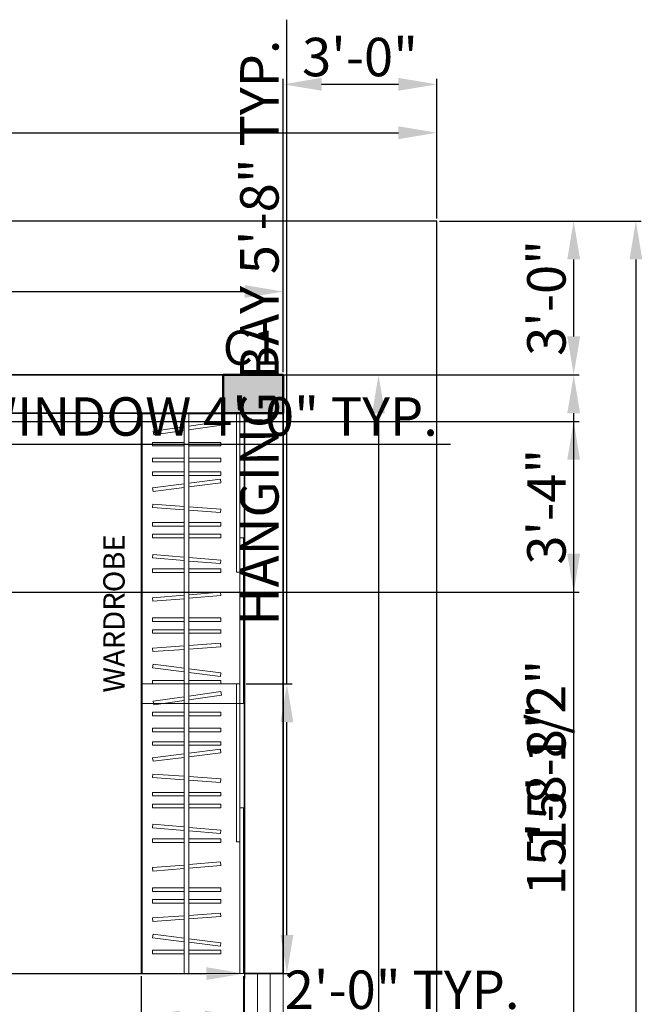
# Model space of a CAD drawing. Units: inches. Extents: x 2621 to 6190, y 513 to 1320.
# Tile 11 of 11: x 3161 to 3306, y 939 to 1169. Entities that reach past the tile are written whole.
import ezdxf

# ---------------------------------------------------------------- set-up
doc = ezdxf.new("R2010")
doc.units = ezdxf.units.IN
for name, color, linetype, lineweight in [('A-ANNO-DIMS', 5, 'Continuous', 18), ('A-ANNO-TEXT', 7, 'Continuous', 18), ('A-FLOR-CASE', 30, 'Continuous', 18), ('A-WALL', 7, 'Continuous', 35), ('C-PROP', 7, 'Continuous', 25), ('columns', 2, 'Continuous', 50), ('S-COLS-IDEN', 2, 'Continuous', 25), ('S-COLS-PATT', 2, 'Continuous', 13), ('window', 172, 'Continuous', 18)]:
    doc.layers.add(name, color=color, linetype=linetype, lineweight=lineweight)
doc.styles.get("Standard").update_dxf_attribs({"font": 'arial.ttf'})
doc.dimstyles.new('ISO-25', dxfattribs={"dimtxt": 9, "dimasz": 9, "dimexe": 1.25, "dimexo": 0.625, "dimtad": 1, "dimlunit": 3, "dimtxsty": 'Standard', "dimcen": 2.5, "dimadec": 0, "dimazin": 0, "dimtfac": 1, "dimtmove": 0, "dimatfit": 3, "dimfxl": 1, "dimarcsym": 0})

# ---------------------------------------------------------------- blocks, each defined once
blk = doc.blocks.new('*D24')
at = {"layer": 'A-ANNO-DIMS', "color": 0, "lineweight": -2, "transparency": 16777216}
for p, q in [((3033.38, 1015.01), (3033.38, 944.49)), ((3213.38, 1015.01), (3213.38, 944.49)), ((3042.38, 945.74), (3204.38, 945.74))]:
    blk.add_line(p, q, dxfattribs=at)
at = {"layer": 'A-ANNO-DIMS', "color": 0, "transparency": 16777216}
for points in [[(3042.38, 947.24), (3042.38, 944.24), (3033.38, 945.74)], [(3204.38, 947.24), (3204.38, 944.24), (3213.38, 945.74)]]:
    blk.add_solid(points, dxfattribs=at)
at = {"layer": 'Defpoints', "color": 0, "transparency": 16777216}
for p in [(3033.38, 1015.63), (3213.38, 1015.63), (3213.38, 945.74)]:
    blk.add_point(p, dxfattribs=at)
at = {"layer": 'A-ANNO-DIMS', "color": 0, "transparency": 16777216, "insert": (3123.38, 950.97), "char_height": 9, "attachment_point": 5}
blk.add_mtext("15'", dxfattribs=at)
blk = doc.blocks.new('*D35')
at = {"layer": 'A-ANNO-DIMS', "color": 0, "lineweight": -2, "transparency": 16777216}
for p, q in [((3223.01, 1085.89), (3245.96, 1085.89)), ((3244.71, 1076.89), (3244.71, 710.89)), ((3223.01, 701.89), (3245.96, 701.89))]:
    blk.add_line(p, q, dxfattribs=at)
at = {"layer": 'A-ANNO-DIMS', "color": 0, "transparency": 16777216}
for points in [[(3243.21, 1076.89), (3246.21, 1076.89), (3244.71, 1085.89)], [(3243.21, 710.89), (3246.21, 710.89), (3244.71, 701.89)]]:
    blk.add_solid(points, dxfattribs=at)
at = {"layer": 'Defpoints', "color": 0, "transparency": 16777216}
for p in [(3222.38, 1085.89), (3222.38, 701.89), (3244.71, 701.89)]:
    blk.add_point(p, dxfattribs=at)
at = {"layer": 'A-ANNO-DIMS', "color": 0, "transparency": 16777216, "insert": (3239.48, 893.89), "char_height": 9, "attachment_point": 5, "rotation": 90}
blk.add_mtext("32'", dxfattribs=at)
blk = doc.blocks.new('*D36')
at = {"layer": 'A-ANNO-DIMS', "color": 0, "lineweight": -2, "transparency": 16777216}
for p, q in [((2778.38, 1086.51), (2778.38, 1106.64)), ((3222.38, 1086.51), (3222.38, 1106.64)), ((2787.38, 1105.39), (3213.38, 1105.39))]:
    blk.add_line(p, q, dxfattribs=at)
at = {"layer": 'A-ANNO-DIMS', "color": 0, "transparency": 16777216}
for points in [[(2787.38, 1106.89), (2787.38, 1103.89), (2778.38, 1105.39)], [(3213.38, 1106.89), (3213.38, 1103.89), (3222.38, 1105.39)]]:
    blk.add_solid(points, dxfattribs=at)
at = {"layer": 'Defpoints', "color": 0, "transparency": 16777216}
for p in [(3222.38, 1105.39), (2778.38, 1085.89), (3222.38, 1085.89)]:
    blk.add_point(p, dxfattribs=at)
at = {"layer": 'A-ANNO-DIMS', "color": 0, "transparency": 16777216, "insert": (3000.38, 1110.61), "char_height": 9, "attachment_point": 5}
blk.add_mtext("37'", dxfattribs=at)
blk = doc.blocks.new('*D38')
at = {"layer": 'A-ANNO-DIMS', "color": 0, "lineweight": -2, "transparency": 16777216}
for p, q in [((2742.38, 1122.51), (2742.38, 1143.81)), ((3258.38, 1122.51), (3258.38, 1143.81)), ((2751.38, 1142.56), (3249.38, 1142.56))]:
    blk.add_line(p, q, dxfattribs=at)
at = {"layer": 'A-ANNO-DIMS', "color": 0, "transparency": 16777216}
for points in [[(2751.38, 1144.06), (2751.38, 1141.06), (2742.38, 1142.56)], [(3249.38, 1144.06), (3249.38, 1141.06), (3258.38, 1142.56)]]:
    blk.add_solid(points, dxfattribs=at)
at = {"layer": 'Defpoints', "color": 0, "transparency": 16777216}
for p in [(3258.38, 1142.56), (2742.38, 1121.89), (3258.38, 1121.89)]:
    blk.add_point(p, dxfattribs=at)
at = {"layer": 'A-ANNO-DIMS', "color": 0, "transparency": 16777216, "insert": (3000.38, 1147.79), "char_height": 9, "attachment_point": 5}
blk.add_mtext("43'", dxfattribs=at)
blk = doc.blocks.new('*D39')
at = {"layer": 'A-ANNO-DIMS', "color": 0, "lineweight": -2, "transparency": 16777216}
for p, q in [((3259.01, 1121.89), (3306.19, 1121.89)), ((3304.94, 1112.89), (3304.94, 561.89)), ((3259.01, 552.89), (3306.19, 552.89))]:
    blk.add_line(p, q, dxfattribs=at)
at = {"layer": 'A-ANNO-DIMS', "color": 0, "transparency": 16777216}
for points in [[(3303.44, 1112.89), (3306.44, 1112.89), (3304.94, 1121.89)], [(3303.44, 561.89), (3306.44, 561.89), (3304.94, 552.89)]]:
    blk.add_solid(points, dxfattribs=at)
at = {"layer": 'Defpoints', "color": 0, "transparency": 16777216}
for p in [(3258.38, 1121.89), (3258.38, 552.89), (3304.94, 552.89)]:
    blk.add_point(p, dxfattribs=at)
at = {"layer": 'A-ANNO-DIMS', "color": 0, "transparency": 16777216, "insert": (3299.73, 837.39), "char_height": 9, "attachment_point": 5, "rotation": 90}
blk.add_mtext('47\'-5"', dxfattribs=at)
blk = doc.blocks.new('WIN-48IN')
for p, q in [((48, 9), (0, 9)), ((0, 9), (0, 0)), ((48, 0), (48, 9)), ((0, 6), (48, 6)), ((0, 3), (48, 3)), ((0, 0), (48, 0))]:
    blk.add_line(p, q)
blk = doc.blocks.new('WARDROBE-HANGING-BAY')
for p, q in [((0, 0), (0, 67.83)), ((0, 67.83), (23.09, 67.83)), ((10.01, 67.78), (10.01, 0)), ((11.13, 0), (11.13, 67.78)), ((23.09, 0), (0, 0))]:
    blk.add_line(p, q)
for points in [[(23.09, 30.8), (23.09, 67.83), (22.26, 67.83), (22.26, 30.8)], [(23.91, 38.78), (23.91, 0), (23.09, 0), (23.09, 38.78)]]:
    blk.add_lwpolyline(points, close=True)
for points in [[(10.01, 64.78), (2.81, 63.75), (2.92, 62.93)], [(11.13, 64.11), (18.75, 65.19), (18.63, 66.01), (11.13, 64.94)], [(2.92, 62.93), (10.01, 63.95)], [(10.01, 61.16), (2.65, 61.16), (2.65, 60.34)], [(2.65, 60.34), (10.01, 60.34)], [(11.13, 60.34), (18.63, 60.34), (18.63, 61.16), (11.13, 61.16)], [(10.01, 57.44), (2.65, 57.44), (2.65, 56.61)], [(2.65, 56.61), (10.01, 56.61)], [(11.13, 56.61), (18.63, 56.61), (18.63, 57.44), (11.13, 57.44)], [(10.01, 54.27), (2.65, 54.27), (2.65, 53.44)], [(2.65, 53.44), (10.01, 53.44)], [(11.13, 53.44), (18.63, 53.44), (18.63, 54.27), (11.13, 54.27)], [(10.01, 51.44), (2.66, 50.5), (2.76, 49.68)], [(11.13, 50.74), (18.62, 51.69), (18.52, 52.51), (11.13, 51.58)], [(2.76, 49.68), (10.01, 50.6)], [(10.01, 46.18), (2.7, 46.71), (2.64, 45.89)], [(11.13, 45.27), (18.58, 44.73), (18.64, 45.56), (11.13, 46.1)], [(2.64, 45.89), (10.01, 45.35)], [(10.01, 42.41), (2.65, 42.41), (2.65, 41.58)], [(2.65, 41.58), (10.01, 41.58)], [(11.13, 41.58), (18.63, 41.58), (18.63, 42.41), (11.13, 42.41)], [(10.01, 39.65), (2.65, 39.65), (2.65, 38.83)], [(11.13, 38.83), (18.63, 38.83), (18.63, 39.65), (11.13, 39.65)], [(2.65, 38.83), (10.01, 38.83)], [(10.01, 34.32), (2.7, 34.93), (2.63, 34.1)], [(2.63, 34.1), (10.01, 33.49)], [(11.13, 33.39), (18.56, 32.78), (18.63, 33.6), (11.13, 34.22)], [(10.01, 31.52), (2.65, 31.52), (2.65, 30.69)], [(2.65, 30.69), (10.01, 30.69)], [(11.13, 30.69), (18.63, 30.69), (18.63, 31.52), (11.13, 31.52)], [(2.63, 24.79), (10.01, 25.4)], [(11.13, 25.5), (18.56, 26.12), (18.63, 25.29), (11.13, 24.67)], [(10.01, 24.57), (2.7, 23.96), (2.63, 24.79)], [(2.65, 20.07), (10.01, 20.07)], [(10.01, 19.24), (2.65, 19.24), (2.65, 20.07)], [(11.13, 20.07), (18.63, 20.07), (18.63, 19.24), (11.13, 19.24)], [(10.01, 16.48), (2.65, 16.48), (2.65, 17.31)], [(2.65, 17.31), (10.01, 17.31)], [(11.13, 17.31), (18.63, 17.31), (18.63, 16.48), (11.13, 16.48)], [(11.13, 13.62), (18.58, 14.16), (18.64, 13.34), (11.13, 12.79)], [(2.64, 13.01), (10.01, 13.54)], [(10.01, 12.71), (2.7, 12.18), (2.64, 13.01)], [(10.01, 7.46), (2.66, 8.39), (2.76, 9.21)], [(2.76, 9.21), (10.01, 8.29)], [(11.13, 8.15), (18.62, 7.2), (18.52, 6.38), (11.13, 7.31)], [(10.01, 4.62), (2.65, 4.62), (2.65, 5.45)], [(2.65, 5.45), (10.01, 5.45)], [(11.13, 5.45), (18.63, 5.45), (18.63, 4.62), (11.13, 4.62)]]:
    blk.add_lwpolyline(points)
blk = doc.blocks.new('*D55')
at = {"layer": 'A-ANNO-DIMS', "color": 0, "lineweight": -2, "transparency": 16777216}
for p, q in [((3089.38, 1076.26), (3089.38, 1068.44)), ((3137.38, 1076.26), (3137.38, 1068.44)), ((3098.38, 1069.69), (3128.38, 1069.69)), ((3137.38, 1069.69), (3261.52, 1069.69))]:
    blk.add_line(p, q, dxfattribs=at)
at = {"layer": 'A-ANNO-DIMS', "color": 0, "transparency": 16777216}
for points in [[(3098.38, 1071.19), (3098.38, 1068.19), (3089.38, 1069.69)], [(3128.38, 1071.19), (3128.38, 1068.19), (3137.38, 1069.69)]]:
    blk.add_solid(points, dxfattribs=at)
at = {"layer": 'Defpoints', "color": 0, "transparency": 16777216}
for p in [(3089.38, 1076.89), (3137.38, 1076.89), (3137.38, 1069.69)]:
    blk.add_point(p, dxfattribs=at)
at = {"layer": 'A-ANNO-DIMS', "color": 0, "transparency": 16777216, "insert": (3203.95, 1074.97), "char_height": 9, "attachment_point": 5}
blk.add_mtext('WINDOW 4\'-0" TYP.', dxfattribs=at)
blk = doc.blocks.new('*D61')
at = {"layer": 'A-ANNO-DIMS', "color": 0, "lineweight": -2, "transparency": 16777216}
for p, q in [((3223.27, 1013.57), (3223.27, 1169.02)), ((3213.72, 1013.57), (3224.52, 1013.57)), ((3223.27, 954.74), (3223.27, 1004.57)), ((3213.72, 945.74), (3224.52, 945.74))]:
    blk.add_line(p, q, dxfattribs=at)
at = {"layer": 'A-ANNO-DIMS', "color": 0, "transparency": 16777216}
for points in [[(3221.77, 1004.57), (3224.77, 1004.57), (3223.27, 1013.57)], [(3221.77, 954.74), (3224.77, 954.74), (3223.27, 945.74)]]:
    blk.add_solid(points, dxfattribs=at)
at = {"layer": 'Defpoints', "color": 0, "transparency": 16777216}
for p in [(3213.1, 1013.57), (3223.27, 1013.57), (3213.1, 945.74)]:
    blk.add_point(p, dxfattribs=at)
at = {"layer": 'A-ANNO-DIMS', "color": 0, "transparency": 16777216, "insert": (3217.99, 1095.79), "char_height": 9, "attachment_point": 5, "rotation": 90}
blk.add_mtext('HANGING BAY 5\'-8" TYP.', dxfattribs=at)
blk = doc.blocks.new('*D62')
at = {"layer": 'A-ANNO-DIMS', "color": 0, "lineweight": -2, "transparency": 16777216}
for p, q in [((3189.19, 945.12), (3189.19, 934.32)), ((3213.1, 945.12), (3213.1, 934.32)), ((3198.19, 935.57), (3204.1, 935.57)), ((3213.1, 935.57), (3278.36, 935.57))]:
    blk.add_line(p, q, dxfattribs=at)
at = {"layer": 'A-ANNO-DIMS', "color": 0, "transparency": 16777216}
for points in [[(3198.19, 937.07), (3198.19, 934.07), (3189.19, 935.57)], [(3204.1, 937.07), (3204.1, 934.07), (3213.1, 935.57)]]:
    blk.add_solid(points, dxfattribs=at)
at = {"layer": 'Defpoints', "color": 0, "transparency": 16777216}
for p in [(3189.19, 945.74), (3213.1, 945.74), (3213.1, 935.57)]:
    blk.add_point(p, dxfattribs=at)
at = {"layer": 'A-ANNO-DIMS', "color": 0, "transparency": 16777216, "insert": (3250.23, 940.79), "char_height": 9, "attachment_point": 5}
blk.add_mtext('2\'-0" TYP.', dxfattribs=at)
blk = doc.blocks.new('*D83')
at = {"layer": 'A-ANNO-DIMS', "color": 0, "lineweight": -2, "transparency": 16777216}
for p, q in [((3028.01, 1085.89), (3291.63, 1085.89)), ((3290.38, 906.39), (3290.38, 1076.89)), ((3028.01, 897.39), (3291.63, 897.39))]:
    blk.add_line(p, q, dxfattribs=at)
at = {"layer": 'A-ANNO-DIMS', "color": 0, "transparency": 16777216}
for points in [[(3288.88, 1076.89), (3291.88, 1076.89), (3290.38, 1085.89)], [(3288.88, 906.39), (3291.88, 906.39), (3290.38, 897.39)]]:
    blk.add_solid(points, dxfattribs=at)
at = {"layer": 'Defpoints', "color": 0, "transparency": 16777216}
for p in [(3027.38, 1085.89), (3290.38, 1085.89), (3027.38, 897.39)]:
    blk.add_point(p, dxfattribs=at)
at = {"layer": 'A-ANNO-DIMS', "color": 0, "transparency": 16777216, "insert": (3285.1, 991.64), "char_height": 9, "attachment_point": 5, "rotation": 90}
blk.add_mtext('15\'-8 1/2"', dxfattribs=at)
blk = doc.blocks.new('*D84')
at = {"layer": 'A-ANNO-DIMS', "color": 0, "lineweight": -2, "transparency": 16777216}
for p, q in [((3223.01, 1085.89), (3291.63, 1085.89)), ((3290.38, 906.74), (3290.38, 1076.89)), ((3223.01, 897.74), (3291.63, 897.74))]:
    blk.add_line(p, q, dxfattribs=at)
at = {"layer": 'A-ANNO-DIMS', "color": 0, "transparency": 16777216}
for points in [[(3288.88, 1076.89), (3291.88, 1076.89), (3290.38, 1085.89)], [(3288.88, 906.74), (3291.88, 906.74), (3290.38, 897.74)]]:
    blk.add_solid(points, dxfattribs=at)
at = {"layer": 'Defpoints', "color": 0, "transparency": 16777216}
for p in [(3222.38, 1085.89), (3290.38, 1085.89), (3222.38, 897.74)]:
    blk.add_point(p, dxfattribs=at)
at = {"layer": 'A-ANNO-DIMS', "color": 0, "transparency": 16777216, "insert": (3285.16, 991.82), "char_height": 9, "attachment_point": 5, "rotation": 90}
blk.add_mtext('15\'-8"', dxfattribs=at)
blk = doc.blocks.new('*D89')
at = {"layer": 'A-ANNO-DIMS', "color": 0, "lineweight": -2, "transparency": 16777216}
for p, q in [((3259.01, 1121.89), (3291.63, 1121.89)), ((3290.38, 1094.89), (3290.38, 1112.89)), ((3223.01, 1085.89), (3291.63, 1085.89))]:
    blk.add_line(p, q, dxfattribs=at)
at = {"layer": 'A-ANNO-DIMS', "color": 0, "transparency": 16777216}
for points in [[(3288.88, 1112.89), (3291.88, 1112.89), (3290.38, 1121.89)], [(3288.88, 1094.89), (3291.88, 1094.89), (3290.38, 1085.89)]]:
    blk.add_solid(points, dxfattribs=at)
at = {"layer": 'Defpoints', "color": 0, "transparency": 16777216}
for p in [(3258.38, 1121.89), (3290.38, 1121.89), (3222.38, 1085.89)]:
    blk.add_point(p, dxfattribs=at)
at = {"layer": 'A-ANNO-DIMS', "color": 0, "transparency": 16777216, "insert": (3285.16, 1103.89), "char_height": 9, "attachment_point": 5, "rotation": 90}
blk.add_mtext('3\'-0"', dxfattribs=at)
blk = doc.blocks.new('*D90')
at = {"layer": 'A-ANNO-DIMS', "color": 0, "lineweight": -2, "transparency": 16777216}
for p, q in [((3222.38, 1086.51), (3222.38, 1155.14)), ((3258.38, 1122.51), (3258.38, 1155.14)), ((3231.38, 1153.89), (3249.38, 1153.89))]:
    blk.add_line(p, q, dxfattribs=at)
at = {"layer": 'A-ANNO-DIMS', "color": 0, "transparency": 16777216}
for points in [[(3231.38, 1155.39), (3231.38, 1152.39), (3222.38, 1153.89)], [(3249.38, 1155.39), (3249.38, 1152.39), (3258.38, 1153.89)]]:
    blk.add_solid(points, dxfattribs=at)
at = {"layer": 'Defpoints', "color": 0, "transparency": 16777216}
for p in [(3258.38, 1153.89), (3258.38, 1121.89), (3222.38, 1085.89)]:
    blk.add_point(p, dxfattribs=at)
at = {"layer": 'A-ANNO-DIMS', "color": 0, "transparency": 16777216, "insert": (3240.38, 1159.11), "char_height": 9, "attachment_point": 5}
blk.add_mtext('3\'-0"', dxfattribs=at)
blk = doc.blocks.new('*D91')
at = {"layer": 'A-ANNO-DIMS', "color": 0, "lineweight": -2, "transparency": 16777216}
for p, q in [((3223.01, 1085.89), (3291.63, 1085.89)), ((3290.38, 629.89), (3290.38, 1076.89)), ((3223.01, 620.89), (3291.63, 620.89))]:
    blk.add_line(p, q, dxfattribs=at)
at = {"layer": 'A-ANNO-DIMS', "color": 0, "transparency": 16777216}
for points in [[(3288.88, 1076.89), (3291.88, 1076.89), (3290.38, 1085.89)], [(3288.88, 629.89), (3291.88, 629.89), (3290.38, 620.89)]]:
    blk.add_solid(points, dxfattribs=at)
at = {"layer": 'Defpoints', "color": 0, "transparency": 16777216}
for p in [(3222.38, 1085.89), (3290.38, 1085.89), (3222.38, 620.89)]:
    blk.add_point(p, dxfattribs=at)
at = {"layer": 'A-ANNO-DIMS', "color": 0, "transparency": 16777216, "insert": (3285.16, 853.39), "char_height": 9, "attachment_point": 5, "rotation": 90}
blk.add_mtext('38\'-9"', dxfattribs=at)
blk = doc.blocks.new('*D103')
at = {"layer": 'A-ANNO-DIMS', "color": 0, "lineweight": -2, "transparency": 16777216}
for p, q in [((2929.85, 1075), (3291.63, 1075)), ((3290.38, 1044.05), (3290.38, 1066)), ((2929.85, 1035.05), (3291.63, 1035.05))]:
    blk.add_line(p, q, dxfattribs=at)
at = {"layer": 'A-ANNO-DIMS', "color": 0, "transparency": 16777216}
for points in [[(3288.88, 1066), (3291.88, 1066), (3290.38, 1075)], [(3288.88, 1044.05), (3291.88, 1044.05), (3290.38, 1035.05)]]:
    blk.add_solid(points, dxfattribs=at)
at = {"layer": 'Defpoints', "color": 0, "transparency": 16777216}
for p in [(2929.23, 1075), (3290.38, 1075), (2929.23, 1035.05)]:
    blk.add_point(p, dxfattribs=at)
at = {"layer": 'A-ANNO-DIMS', "color": 0, "transparency": 16777216, "insert": (3285.16, 1055.03), "char_height": 9, "attachment_point": 5, "rotation": 90}
blk.add_mtext('3\'-4"', dxfattribs=at)

msp = doc.modelspace()

# ---------------------------------------------------------------- hatches: boundary and pattern name
at = {"layer": 'S-COLS-PATT'}
h = msp.add_hatch(color=256, dxfattribs=at)
h.dxf.hatch_style = 1
h.paths.add_polyline_path([(2787.381, 1085.89), (2778.381, 1085.89), (2778.381, 1071.89), (2787.381, 1071.89)])
h.paths.add_polyline_path([(3222.381, 1085.89), (3208.381, 1085.89), (3208.381, 1076.89), (3222.381, 1076.89)])
h.paths.add_polyline_path([(3041.381, 1085.89), (3027.381, 1085.89), (3027.381, 1076.89), (3041.381, 1076.89)])
h.paths.add_polyline_path([(2916.381, 1085.89), (2907.381, 1085.89), (2907.381, 1076.89), (2916.381, 1076.89)])
h.paths.add_polyline_path([(2916.381, 1076.89), (2913.381, 1076.89), (2913.381, 1071.89), (2916.381, 1071.89)])
h.paths.add_polyline_path([(2913.381, 1076.89), (2907.381, 1076.89), (2907.381, 1071.89), (2913.381, 1071.89)])
h.paths.add_polyline_path([(2787.381, 896.89), (2778.381, 896.89), (2778.381, 882.89), (2787.381, 882.89)])
h.paths.add_polyline_path([(2924.221, 898.241), (2910.221, 898.241), (2910.221, 889.241), (2924.221, 889.241)])
h.paths.add_polyline_path([(3036.381, 896.89), (3033.381, 896.89), (3027.381, 897.385), (3027.381, 883.385), (3033.381, 883.385), (3033.381, 890.89), (3036.381, 890.89)])
h.paths.add_polyline_path([(3036.381, 890.89), (3033.381, 890.89), (3033.381, 883.385), (3036.381, 883.385)], flags=17)
h.paths.add_polyline_path([(3222.381, 897.745), (3213.381, 897.745), (3213.381, 883.745), (3222.381, 883.745)])
h.paths.add_polyline_path([(3222.381, 710.89), (3208.381, 710.89), (3208.381, 701.89), (3222.381, 701.89)])
h.paths.add_polyline_path([(3039.318, 710.89), (3021.318, 710.89), (3021.318, 701.89), (3039.318, 701.89)])
h.paths.add_polyline_path([(2796.381, 710.89), (2778.381, 710.89), (2778.381, 701.89), (2796.381, 701.89)])

# ---------------------------------------------------------------- linework, layer by layer
at = {"layer": 'A-FLOR-CASE'}
for p, q in [((3189.381, 945.745), (3189.381, 1076.89)), ((3213.381, 945.745), (3189.381, 945.745))]:
    msp.add_line(p, q, dxfattribs=at)
at = {"layer": 'A-WALL'}
for p, q in [((3222.381, 1085.89), (3137.381, 1085.89)), ((3222.381, 945.745), (3222.381, 1085.89)), ((3213.381, 1076.89), (3137.381, 1076.89)), ((3213.381, 945.745), (3213.381, 1076.89)), ((3213.381, 945.745), (3222.381, 945.745))]:
    msp.add_line(p, q, dxfattribs=at)
at = {"layer": 'C-PROP'}
msp.add_lwpolyline([(3258.381, 552.89), (3258.381, 1121.89), (2742.381, 1121.89), (2718.381, 552.89)], close=True, dxfattribs=at)
at = {"layer": 'columns'}
msp.add_lwpolyline([(3208.381, 1076.89), (3208.381, 1085.89), (3222.381, 1085.89), (3222.381, 1076.89)], close=True, dxfattribs=at)

# ---------------------------------------------------------------- block references
at = {"layer": 'A-FLOR-CASE'}
for p in [(3189.186, 1008.921), (3189.186, 945.745)]:
    msp.add_blockref('WARDROBE-HANGING-BAY', p, dxfattribs=at)
at = {"layer": 'window', "rotation": 89.99999999999805}
msp.add_blockref('WIN-48IN', (3222.381, 897.745), dxfattribs=at)

# ---------------------------------------------------------------- texts
at = {"layer": 'A-ANNO-TEXT', "insert": (3180.294, 1011.498), "char_height": 5, "attachment_point": 1, "rotation": 90}
msp.add_mtext_dynamic_manual_height_columns('WARDROBE', width=41.95014, gutter_width=12.5, heights=[0], dxfattribs=at)
at = {"layer": 'S-COLS-IDEN', "insert": (3208.285, 1096.24), "char_height": 8, "attachment_point": 1}
msp.add_mtext_dynamic_manual_height_columns('C1', width=53.01391, gutter_width=12.5, heights=[0], dxfattribs=at)

# ---------------------------------------------------------------- dimensions: what is measured, and where the dimension line sits
at = {"layer": 'A-ANNO-DIMS'}
dim = msp.add_linear_dim(base=(3223.272, 1013.57), p1=(3213.098, 945.745), p2=(3213.098, 1013.57), angle=90, text='HANGING BAY <> TYP.', dimstyle='ISO-25', override={"dimdec": 1, "dimlfac": 1, "dimrnd": 0, "dimzin": 1, "dimdsep": 46, "dimlunit": 4, "dimfrac": 2}, dxfattribs=at)
dim.commit()
dim.dimension.update_dxf_attribs({"geometry": '*D61', "text_midpoint": (3217.994, 1095.794)})
for base, p1, p2, override, picture, middle in [((3258.381, 1153.89), (3222.381, 1085.89), (3258.381, 1121.89), {"dimdec": 1, "dimlfac": 1, "dimrnd": 0, "dimzin": 1, "dimdsep": 46, "dimlunit": 4, "dimfrac": 2}, '*D90', (3240.381, 1159.113)), ((3258.381, 1142.564), (2742.381, 1121.89), (3258.381, 1121.89), {"dimclrd": 0, "dimclre": 0, "dimclrt": 0}, '*D38', (3000.381, 1147.788)), ((3222.381, 1105.387), (2778.381, 1085.89), (3222.381, 1085.89), {"dimclrd": 0, "dimclre": 0, "dimclrt": 0}, '*D36', (3000.381, 1110.61)), ((3213.381, 945.745), (3033.381, 1015.632), (3213.381, 1015.632), {"dimclrd": 0, "dimclre": 0, "dimclrt": 0}, '*D24', (3123.381, 950.965))]:
    dim = msp.add_linear_dim(base=base, p1=p1, p2=p2, dimstyle='ISO-25', override=override, dxfattribs=at)
    dim.commit()
    dim.dimension.update_dxf_attribs({"geometry": picture, "text_midpoint": middle})
for base, p1, p2, override, picture, middle in [((3290.381, 1121.89), (3222.381, 1085.89), (3258.381, 1121.89), {"dimdec": 1, "dimlfac": 1, "dimrnd": 0, "dimzin": 1, "dimdsep": 46, "dimlunit": 4, "dimfrac": 2}, '*D89', (3285.158, 1103.89)), ((3304.936, 552.89), (3258.381, 1121.89), (3258.381, 552.89), {"dimclrd": 0, "dimclre": 0, "dimclrt": 0}, '*D39', (3299.735, 837.39)), ((3290.381, 1085.89), (3027.381, 897.385), (3027.381, 1085.89), {"dimdec": 1, "dimlfac": 1, "dimrnd": 0, "dimzin": 1, "dimdsep": 46, "dimlunit": 4, "dimfrac": 2}, '*D83', (3285.103, 991.637)), ((3290.381, 1085.89), (3222.381, 897.745), (3222.381, 1085.89), {"dimdec": 1, "dimlfac": 1, "dimrnd": 0, "dimzin": 1, "dimdsep": 46, "dimlunit": 4, "dimfrac": 2}, '*D84', (3285.161, 991.817)), ((3290.381, 1085.89), (3222.381, 620.89), (3222.381, 1085.89), {"dimdec": 1, "dimlfac": 1, "dimrnd": 0, "dimzin": 1, "dimdsep": 46, "dimlunit": 4, "dimfrac": 2}, '*D91', (3285.158, 853.39)), ((3290.381, 1075.001), (2929.225, 1035.049), (2929.225, 1075.001), {"dimdec": 1, "dimlfac": 1, "dimrnd": 0, "dimzin": 1, "dimdsep": 46, "dimlunit": 4, "dimfrac": 2}, '*D103', (3285.158, 1055.025))]:
    dim = msp.add_linear_dim(base=base, p1=p1, p2=p2, angle=90, dimstyle='ISO-25', override=override, dxfattribs=at)
    dim.commit()
    dim.dimension.update_dxf_attribs({"geometry": picture, "text_midpoint": middle})
for base, p1, p2, text, picture, middle in [((3137.381, 1069.69), (3089.381, 1076.89), (3137.381, 1076.89), 'WINDOW <> TYP.', '*D55', (3203.95, 1074.971)), ((3213.098, 935.571), (3189.186, 945.745), (3213.098, 945.745), '<> TYP.', '*D62', (3250.23, 940.791))]:
    dim = msp.add_linear_dim(base=base, p1=p1, p2=p2, text=text, dimstyle='ISO-25', override={"dimdec": 1, "dimlfac": 1, "dimrnd": 0, "dimzin": 1, "dimdsep": 46, "dimlunit": 4, "dimfrac": 2}, dxfattribs=at)
    dim.commit()
    dim.dimension.update_dxf_attribs({"geometry": picture, "text_midpoint": middle})
dim = msp.add_linear_dim(base=(3244.707, 701.89), p1=(3222.381, 1085.89), p2=(3222.381, 701.89), angle=90, dimstyle='ISO-25', override={"dimclrd": 0, "dimclre": 0, "dimclrt": 0}, dxfattribs=at)
dim.commit()
dim.dimension.update_dxf_attribs({"geometry": '*D35', "text_midpoint": (3244.707, 893.89), "dimtype": 160})

doc.saveas('drawing.dxf')
